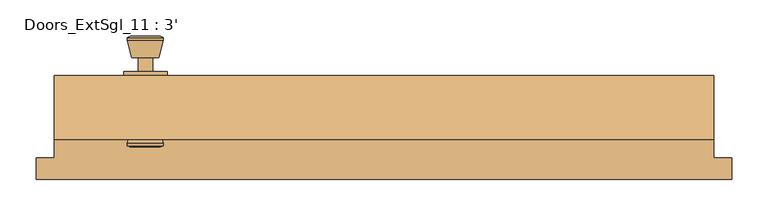
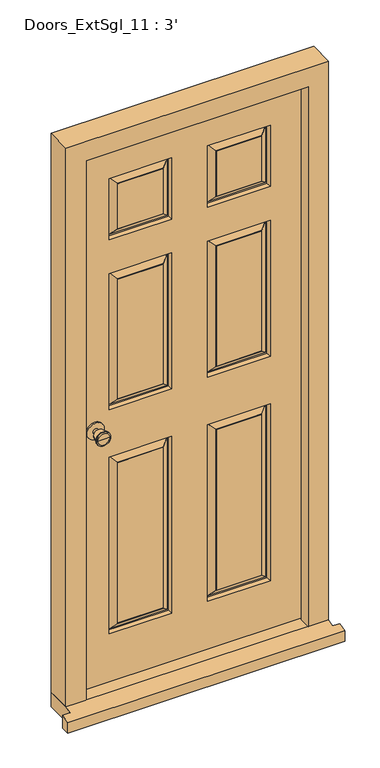
"""IFC4 building model written with IfcOpenShell, lengths in millimetres: door geometry, Doors_ExtSgl_11 : 3'."""

from ifc_helpers import new_model, si_unit, point, frame, frame_2d, origin, place, context, project, spatial, polyline, circle_curve, trimmed, segment, composite_curve, outline, extrude, faceted_brep, source, transform, mapped, element, save
from ifc_brep_helpers import plane_surface, cylinder_surface, revolved_surface, advanced_brep


def doors_extsgl_11_3_1bca8958(model_context):
    return source(origin(), model_context, "Body", "SolidModel", [
        advanced_brep(
        [(-330.7, 51.42, 1000.0), (-340.7, 51.42, 1000.0), (-320.7, 51.42, 1000.0), (-310.2241324, 100.42, 1000.0), (-351.1758676, 100.42, 1000.0), (-330.7, 100.42, 1000.0), (-305.7, 98.5921319, 1000.0), (-355.7, 98.5921319, 1000.0), (-305.7, 95.1284537, 1000.0), (-355.7, 95.1284537, 1000.0), (-312.063764, 70.42, 1000.0), (-349.336236, 70.42, 1000.0), (-320.7, 70.42, 1000.0), (-340.7, 70.42, 1000.0)],
        [
            (0, 1),
            (1, 2, circle_curve(frame((-330.7, 51.42, 1000.0), z_axis=(0.0, -1.0, 0.0), x_axis=(-1.0, 0.0, 0.0)), 10.0)),
            (2, 0),
            (2, 1, circle_curve(frame((-330.7, 51.42, 1000.0), z_axis=(0.0, -1.0, 0.0), x_axis=(-1.0, 0.0, 0.0)), 10.0)),
            (3, 4, circle_curve(frame((-330.7, 100.42, 1000.0), z_axis=(0.0, 1.0, 0.0), x_axis=(-1.0, 0.0, 0.0)), 20.4758676)),
            (4, 5),
            (5, 3),
            (4, 3, circle_curve(frame((-330.7, 100.42, 1000.0), z_axis=(0.0, 1.0, 0.0), x_axis=(-1.0, 0.0, 0.0)), 20.4758676)),
            (6, 7, circle_curve(frame((-330.7, 98.5921319, 1000.0), z_axis=(0.0, 1.0, 0.0), x_axis=(-1.0, 0.0, 0.0)), 25.0)),
            (7, 4),
            (3, 6),
            (7, 6, circle_curve(frame((-330.7, 98.5921319, 1000.0), z_axis=(0.0, 1.0, 0.0), x_axis=(-1.0, 0.0, 0.0)), 25.0)),
            (8, 9, circle_curve(frame((-330.7, 95.1284537, 1000.0), z_axis=(0.0, 1.0, 0.0), x_axis=(-1.0, 0.0, 0.0)), 25.0)),
            (9, 7),
            (6, 8),
            (9, 8, circle_curve(frame((-330.7, 95.1284537, 1000.0), z_axis=(0.0, 1.0, 0.0), x_axis=(-1.0, 0.0, 0.0)), 25.0)),
            (10, 11, circle_curve(frame((-330.7, 70.42, 1000.0), z_axis=(0.0, 1.0, 0.0), x_axis=(-1.0, 0.0, 0.0)), 18.636236)),
            (11, 9),
            (8, 10),
            (11, 10, circle_curve(frame((-330.7, 70.42, 1000.0), z_axis=(0.0, 1.0, 0.0), x_axis=(-1.0, 0.0, 0.0)), 18.636236)),
            (12, 13, circle_curve(frame((-330.7, 70.42, 1000.0), z_axis=(0.0, 1.0, 0.0), x_axis=(-1.0, 0.0, 0.0)), 10.0)),
            (13, 11),
            (10, 12),
            (13, 12, circle_curve(frame((-330.7, 70.42, 1000.0), z_axis=(0.0, 1.0, 0.0), x_axis=(-1.0, 0.0, 0.0)), 10.0)),
            (1, 13),
            (12, 2),
        ],
        [
            plane_surface(frame((-330.7, 51.42, 1000.0), z_axis=(0.0, -1.0, 0.0), x_axis=(-1.0, 0.0, 0.0))),
            plane_surface(frame((-330.7, 100.42, 1000.0), z_axis=(0.0, 1.0, 0.0), x_axis=(-1.0, 0.0, 0.0))),
            revolved_surface(polyline([(-351.1758676, 100.42, 1000.0), (-355.7, 98.5921319, 1000.0)]), (-330.7, 51.42, 1000.0), (0.0, -1.0, 0.0)),
            cylinder_surface(frame((-330.7, 51.42, 1000.0), z_axis=(0.0, -1.0, 0.0), x_axis=(-1.0, 0.0, 0.0)), 25.0),
            revolved_surface(polyline([(-355.7, 95.1284537, 1000.0), (-349.336236, 70.42, 1000.0)]), (-330.7, 51.42, 1000.0), (0.0, -1.0, 0.0)),
            plane_surface(frame((-330.7, 70.42, 1000.0), z_axis=(0.0, -1.0, 0.0), x_axis=(-1.0, 0.0, 0.0))),
            cylinder_surface(frame((-330.7, 51.42, 1000.0), z_axis=(0.0, -1.0, 0.0), x_axis=(-1.0, 0.0, 0.0)), 10.0),
        ],
        [
            (0, [[1, 2, 3]]),
            (0, [[-3, 4, -1]]),
            (1, [[5, 6, 7]]),
            (1, [[8, -7, -6]]),
            (2, [[9, 10, -5, 11]]),
            (2, [[12, -11, -8, -10]]),
            (3, [[13, 14, -9, 15]]),
            (3, [[16, -15, -12, -14]]),
            (4, [[17, 18, -13, 19]]),
            (4, [[20, -19, -16, -18]]),
            (5, [[21, 22, -17, 23]]),
            (5, [[24, -23, -20, -22]]),
            (6, [[-2, 25, -21, 26]]),
            (6, [[-4, -26, -24, -25]]),
        ],
    ),
        extrude(outline(composite_curve([segment(trimmed(circle_curve(frame_2d((1000.0, -330.7)), 30.0), [point((1000.0, -360.7))], [point((1000.0, -300.7))], False, "CARTESIAN"), True, "CONTINUOUS"), segment(trimmed(circle_curve(frame_2d((1000.0, -330.7)), 30.0), [point((1000.0, -300.7))], [point((1000.0, -360.7))], False, "CARTESIAN"), True, "CONTINUOUS")], self_intersect=False)), frame((0.0, 45.42, 0.0), z_axis=(0.0, 1.0, 0.0), x_axis=(0.0, 0.0, 1.0)), (0.0, 0.0, 1.0), 6.0),
        advanced_brep(
        [(-330.7, -4.58, 1000.0), (-320.7, -4.58, 1000.0), (-340.7, -4.58, 1000.0), (-310.2241324, -53.58, 1000.0), (-330.7, -53.58, 1000.0), (-351.1758676, -53.58, 1000.0), (-305.7, -51.7521319, 1000.0), (-355.7, -51.7521319, 1000.0), (-305.7, -48.2884537, 1000.0), (-355.7, -48.2884537, 1000.0), (-312.063764, -23.58, 1000.0), (-349.336236, -23.58, 1000.0), (-320.7, -23.58, 1000.0), (-340.7, -23.58, 1000.0)],
        [
            (0, 1),
            (1, 2, circle_curve(frame((-330.7, -4.58, 1000.0), z_axis=(0.0, 1.0, 0.0), x_axis=(-1.0, 0.0, 0.0)), 10.0)),
            (2, 0),
            (2, 1, circle_curve(frame((-330.7, -4.58, 1000.0), z_axis=(0.0, 1.0, 0.0), x_axis=(-1.0, 0.0, 0.0)), 10.0)),
            (3, 4),
            (4, 5),
            (5, 3, circle_curve(frame((-330.7, -53.58, 1000.0), z_axis=(0.0, -1.0, 0.0), x_axis=(-1.0, 0.0, 0.0)), 20.4758676)),
            (3, 5, circle_curve(frame((-330.7, -53.58, 1000.0), z_axis=(0.0, -1.0, 0.0), x_axis=(-1.0, 0.0, 0.0)), 20.4758676)),
            (6, 3),
            (5, 7),
            (7, 6, circle_curve(frame((-330.7, -51.7521319, 1000.0), z_axis=(0.0, -1.0, 0.0), x_axis=(-1.0, 0.0, 0.0)), 25.0)),
            (6, 7, circle_curve(frame((-330.7, -51.7521319, 1000.0), z_axis=(0.0, -1.0, 0.0), x_axis=(-1.0, 0.0, 0.0)), 25.0)),
            (8, 6),
            (7, 9),
            (9, 8, circle_curve(frame((-330.7, -48.2884537, 1000.0), z_axis=(0.0, -1.0, 0.0), x_axis=(-1.0, 0.0, 0.0)), 25.0)),
            (8, 9, circle_curve(frame((-330.7, -48.2884537, 1000.0), z_axis=(0.0, -1.0, 0.0), x_axis=(-1.0, 0.0, 0.0)), 25.0)),
            (10, 8),
            (9, 11),
            (11, 10, circle_curve(frame((-330.7, -23.58, 1000.0), z_axis=(0.0, -1.0, 0.0), x_axis=(-1.0, 0.0, 0.0)), 18.636236)),
            (10, 11, circle_curve(frame((-330.7, -23.58, 1000.0), z_axis=(0.0, -1.0, 0.0), x_axis=(-1.0, 0.0, 0.0)), 18.636236)),
            (12, 10),
            (11, 13),
            (13, 12, circle_curve(frame((-330.7, -23.58, 1000.0), z_axis=(0.0, -1.0, 0.0), x_axis=(-1.0, 0.0, 0.0)), 10.0)),
            (12, 13, circle_curve(frame((-330.7, -23.58, 1000.0), z_axis=(0.0, -1.0, 0.0), x_axis=(-1.0, 0.0, 0.0)), 10.0)),
            (1, 12),
            (13, 2),
        ],
        [
            plane_surface(frame((-330.7, -4.58, 1000.0), z_axis=(0.0, 1.0, 0.0), x_axis=(-1.0, 0.0, 0.0))),
            plane_surface(frame((-330.7, -53.58, 1000.0), z_axis=(0.0, -1.0, 0.0), x_axis=(-1.0, 0.0, 0.0))),
            revolved_surface(polyline([(-351.1758676, -53.58, 1000.0), (-355.7, -51.7521319, 1000.0)]), (-330.7, -4.58, 1000.0), (0.0, 1.0, 0.0)),
            cylinder_surface(frame((-330.7, -4.58, 1000.0), z_axis=(0.0, 1.0, 0.0), x_axis=(-1.0, 0.0, 0.0)), 25.0),
            revolved_surface(polyline([(-355.7, -48.2884537, 1000.0), (-349.336236, -23.58, 1000.0)]), (-330.7, -4.58, 1000.0), (0.0, 1.0, 0.0)),
            plane_surface(frame((-330.7, -23.58, 1000.0), z_axis=(0.0, 1.0, 0.0), x_axis=(-1.0, 0.0, 0.0))),
            cylinder_surface(frame((-330.7, -4.58, 1000.0), z_axis=(0.0, 1.0, 0.0), x_axis=(-1.0, 0.0, 0.0)), 10.0),
        ],
        [
            (0, [[1, 2, 3]]),
            (0, [[-3, 4, -1]]),
            (1, [[5, 6, 7]]),
            (1, [[-6, -5, 8]]),
            (2, [[9, -7, 10, 11]]),
            (2, [[-10, -8, -9, 12]]),
            (3, [[13, -11, 14, 15]]),
            (3, [[-14, -12, -13, 16]]),
            (4, [[17, -15, 18, 19]]),
            (4, [[-18, -16, -17, 20]]),
            (5, [[21, -19, 22, 23]]),
            (5, [[-22, -20, -21, 24]]),
            (6, [[25, -23, 26, -2]]),
            (6, [[-26, -24, -25, -4]]),
        ],
    ),
        extrude(outline(composite_curve([segment(trimmed(circle_curve(frame_2d((1000.0, -330.7)), 30.0), [point((1000.0, -360.7))], [point((1000.0, -300.7))], False, "CARTESIAN"), True, "CONTINUOUS"), segment(trimmed(circle_curve(frame_2d((1000.0, -330.7)), 30.0), [point((1000.0, -300.7))], [point((1000.0, -360.7))], False, "CARTESIAN"), True, "CONTINUOUS")], self_intersect=False)), frame((0.0, -4.58, 0.0), z_axis=(0.0, 1.0, 0.0), x_axis=(0.0, 0.0, 1.0)), (0.0, 0.0, 1.0), 6.0),
        faceted_brep([(386.7, -43.58, 54.5), (386.7, -1.58, 54.5), (408.7, -1.58, 54.5), (408.7, 45.42, 54.5), (457.2, 45.42, 54.5), (457.2, -43.58, 54.5), (457.2, -43.58, 2110.0), (-457.2, -43.58, 2110.0), (-457.2, -43.58, 54.5), (-386.7, -43.58, 54.5), (-386.7, -43.58, 2039.5), (386.7, -43.58, 2039.5), (457.2, 45.42, 2110.0), (408.7, 45.42, 2061.5), (-408.7, 45.42, 2061.5), (-408.7, 45.42, 54.5), (-457.2, 45.42, 54.5), (-457.2, 45.42, 2110.0), (408.7, -1.58, 2061.5), (386.7, -1.58, 2039.5), (-386.7, -1.58, 2039.5), (-386.7, -1.58, 54.5), (-408.7, -1.58, 54.5), (-408.7, -1.58, 2061.5)], [[[0, 1, 2, 3, 4, 5]], [[5, 6, 7, 8, 9, 10, 11, 0]], [[4, 12, 6, 5]], [[3, 13, 14, 15, 16, 17, 12, 4]], [[2, 18, 13, 3]], [[1, 19, 20, 21, 22, 23, 18, 2]], [[0, 11, 19, 1]], [[9, 21, 20, 10]], [[8, 16, 15, 22, 21, 9]], [[7, 17, 16, 8]], [[14, 23, 22, 15]], [[6, 12, 17, 7]], [[13, 18, 23, 14]], [[10, 20, 19, 11]]]),
        faceted_brep([(405.7, 45.42, 58.5), (-406.6250294, 45.42, 58.5), (-406.6250294, 45.42, 2058.5), (405.7, 45.42, 2058.5), (-62.5, 45.42, 883.5), (-280.7, 45.42, 883.5), (-280.7, 45.42, 233.5), (-62.5, 45.42, 233.5), (280.7, 45.42, 883.5), (62.5, 45.42, 883.5), (62.5, 45.42, 233.5), (280.7, 45.42, 233.5), (-62.5, 45.42, 1558.5), (-280.7, 45.42, 1558.5), (-280.7, 45.42, 1058.5), (-62.5, 45.42, 1058.5), (280.7, 45.42, 1558.5), (62.5, 45.42, 1558.5), (62.5, 45.42, 1058.5), (280.7, 45.42, 1058.5), (-62.5, 45.42, 1908.5), (-280.7, 45.42, 1908.5), (-280.7, 45.42, 1683.5), (-62.5, 45.42, 1683.5), (62.5, 45.42, 1683.5), (280.7, 45.42, 1683.5), (280.7, 45.42, 1908.5), (62.5, 45.42, 1908.5), (-92.5, 45.42, 263.5), (-250.7, 45.42, 263.5), (-250.7, 45.42, 853.5), (-92.5, 45.42, 853.5), (250.7, 45.42, 263.5), (92.5, 45.42, 263.5), (92.5, 45.42, 853.5), (250.7, 45.42, 853.5), (-92.5, 45.42, 1088.5), (-250.7, 45.42, 1088.5), (-250.7, 45.42, 1528.5), (-92.5, 45.42, 1528.5), (250.7, 45.42, 1088.5), (92.5, 45.42, 1088.5), (92.5, 45.42, 1528.5), (250.7, 45.42, 1528.5), (-92.5, 45.42, 1713.5), (-250.7, 45.42, 1713.5), (-250.7, 45.42, 1878.5), (-92.5, 45.42, 1878.5), (92.5, 45.42, 1878.5), (250.7, 45.42, 1878.5), (250.7, 45.42, 1713.5), (92.5, 45.42, 1713.5), (405.7, 1.42, 58.5), (405.7, 1.42, 2058.5), (-406.6250294, 1.42, 2058.5), (-406.6250294, 1.42, 58.5), (62.5, 1.42, 883.5), (280.7, 1.42, 883.5), (280.7, 1.42, 233.5), (62.5, 1.42, 233.5), (-280.7, 1.42, 883.5), (-62.5, 1.42, 883.5), (-62.5, 1.42, 233.5), (-280.7, 1.42, 233.5), (62.5, 1.42, 1558.5), (280.7, 1.42, 1558.5), (280.7, 1.42, 1058.5), (62.5, 1.42, 1058.5), (-280.7, 1.42, 1558.5), (-62.5, 1.42, 1558.5), (-62.5, 1.42, 1058.5), (-280.7, 1.42, 1058.5), (62.5, 1.42, 1908.5), (280.7, 1.42, 1908.5), (280.7, 1.42, 1683.5), (62.5, 1.42, 1683.5), (-280.7, 1.42, 1908.5), (-62.5, 1.42, 1908.5), (-62.5, 1.42, 1683.5), (-280.7, 1.42, 1683.5), (92.5, 1.42, 263.5), (250.7, 1.42, 263.5), (250.7, 1.42, 853.5), (92.5, 1.42, 853.5), (-250.7, 1.42, 263.5), (-92.5, 1.42, 263.5), (-92.5, 1.42, 853.5), (-250.7, 1.42, 853.5), (92.5, 1.42, 1088.5), (250.7, 1.42, 1088.5), (250.7, 1.42, 1528.5), (92.5, 1.42, 1528.5), (-250.7, 1.42, 1088.5), (-92.5, 1.42, 1088.5), (-92.5, 1.42, 1528.5), (-250.7, 1.42, 1528.5), (92.5, 1.42, 1713.5), (250.7, 1.42, 1713.5), (250.7, 1.42, 1878.5), (92.5, 1.42, 1878.5), (-250.7, 1.42, 1713.5), (-92.5, 1.42, 1713.5), (-92.5, 1.42, 1878.5), (-250.7, 1.42, 1878.5), (65.5, 16.42, 880.5), (65.5, 16.42, 236.5), (90.5, 2.42, 855.5), (70.5, 16.42, 875.5), (70.5, 16.42, 241.5), (90.5, 2.42, 261.5), (92.5, 2.42, 853.5), (92.5, 2.42, 263.5), (277.7, 16.42, 236.5), (272.7, 16.42, 241.5), (252.7, 2.42, 261.5), (250.7, 2.42, 263.5), (277.7, 16.42, 880.5), (272.7, 16.42, 875.5), (252.7, 2.42, 855.5), (250.7, 2.42, 853.5), (-277.7, 16.42, 880.5), (-277.7, 16.42, 236.5), (-252.7, 2.42, 855.5), (-272.7, 16.42, 875.5), (-272.7, 16.42, 241.5), (-252.7, 2.42, 261.5), (-250.7, 2.42, 853.5), (-250.7, 2.42, 263.5), (-65.5, 16.42, 236.5), (-70.5, 16.42, 241.5), (-90.5, 2.42, 261.5), (-92.5, 2.42, 263.5), (-65.5, 16.42, 880.5), (-70.5, 16.42, 875.5), (-90.5, 2.42, 855.5), (-92.5, 2.42, 853.5), (-92.5, 44.42, 263.5), (-92.5, 44.42, 853.5), (-70.5, 30.42, 241.5), (-90.5, 44.42, 261.5), (-90.5, 44.42, 855.5), (-70.5, 30.42, 875.5), (-65.5, 30.42, 236.5), (-65.5, 30.42, 880.5), (-250.7, 44.42, 853.5), (-252.7, 44.42, 855.5), (-272.7, 30.42, 875.5), (-277.7, 30.42, 880.5), (-250.7, 44.42, 263.5), (-252.7, 44.42, 261.5), (-272.7, 30.42, 241.5), (-277.7, 30.42, 236.5), (277.7, 30.42, 880.5), (277.7, 30.42, 236.5), (252.7, 44.42, 855.5), (272.7, 30.42, 875.5), (272.7, 30.42, 241.5), (252.7, 44.42, 261.5), (250.7, 44.42, 853.5), (250.7, 44.42, 263.5), (65.5, 30.42, 236.5), (70.5, 30.42, 241.5), (90.5, 44.42, 261.5), (92.5, 44.42, 263.5), (65.5, 30.42, 880.5), (70.5, 30.42, 875.5), (90.5, 44.42, 855.5), (92.5, 44.42, 853.5), (92.5, 2.42, 1088.5), (92.5, 2.42, 1528.5), (70.5, 16.42, 1066.5), (90.5, 2.42, 1086.5), (90.5, 2.42, 1530.5), (70.5, 16.42, 1550.5), (65.5, 16.42, 1061.5), (65.5, 16.42, 1555.5), (250.7, 2.42, 1528.5), (252.7, 2.42, 1530.5), (272.7, 16.42, 1550.5), (277.7, 16.42, 1555.5), (250.7, 2.42, 1088.5), (252.7, 2.42, 1086.5), (272.7, 16.42, 1066.5), (277.7, 16.42, 1061.5), (-250.7, 2.42, 1088.5), (-250.7, 2.42, 1528.5), (-272.7, 16.42, 1066.5), (-252.7, 2.42, 1086.5), (-252.7, 2.42, 1530.5), (-272.7, 16.42, 1550.5), (-277.7, 16.42, 1061.5), (-277.7, 16.42, 1555.5), (-92.5, 2.42, 1528.5), (-90.5, 2.42, 1530.5), (-70.5, 16.42, 1550.5), (-65.5, 16.42, 1555.5), (-92.5, 2.42, 1088.5), (-90.5, 2.42, 1086.5), (-70.5, 16.42, 1066.5), (-65.5, 16.42, 1061.5), (-92.5, 44.42, 1088.5), (-92.5, 44.42, 1528.5), (-70.5, 30.42, 1066.5), (-90.5, 44.42, 1086.5), (-90.5, 44.42, 1530.5), (-70.5, 30.42, 1550.5), (-65.5, 30.42, 1061.5), (-65.5, 30.42, 1555.5), (-250.7, 44.42, 1528.5), (-252.7, 44.42, 1530.5), (-272.7, 30.42, 1550.5), (-277.7, 30.42, 1555.5), (-250.7, 44.42, 1088.5), (-252.7, 44.42, 1086.5), (-272.7, 30.42, 1066.5), (-277.7, 30.42, 1061.5), (277.7, 30.42, 1555.5), (277.7, 30.42, 1061.5), (252.7, 44.42, 1530.5), (272.7, 30.42, 1550.5), (272.7, 30.42, 1066.5), (252.7, 44.42, 1086.5), (250.7, 44.42, 1528.5), (250.7, 44.42, 1088.5), (65.5, 30.42, 1061.5), (70.5, 30.42, 1066.5), (90.5, 44.42, 1086.5), (92.5, 44.42, 1088.5), (65.5, 30.42, 1555.5), (70.5, 30.42, 1550.5), (90.5, 44.42, 1530.5), (92.5, 44.42, 1528.5), (92.5, 2.42, 1713.5), (92.5, 2.42, 1878.5), (70.5, 16.42, 1691.5), (90.5, 2.42, 1711.5), (90.5, 2.42, 1880.5), (70.5, 16.42, 1900.5), (65.5, 16.42, 1686.5), (65.5, 16.42, 1905.5), (250.7, 2.42, 1878.5), (252.7, 2.42, 1880.5), (272.7, 16.42, 1900.5), (277.7, 16.42, 1905.5), (250.7, 2.42, 1713.5), (252.7, 2.42, 1711.5), (272.7, 16.42, 1691.5), (277.7, 16.42, 1686.5), (-250.7, 2.42, 1713.5), (-250.7, 2.42, 1878.5), (-272.7, 16.42, 1691.5), (-252.7, 2.42, 1711.5), (-252.7, 2.42, 1880.5), (-272.7, 16.42, 1900.5), (-277.7, 16.42, 1686.5), (-277.7, 16.42, 1905.5), (-92.5, 2.42, 1878.5), (-90.5, 2.42, 1880.5), (-70.5, 16.42, 1900.5), (-65.5, 16.42, 1905.5), (-92.5, 2.42, 1713.5), (-90.5, 2.42, 1711.5), (-70.5, 16.42, 1691.5), (-65.5, 16.42, 1686.5), (-92.5, 44.42, 1713.5), (-92.5, 44.42, 1878.5), (-70.5, 30.42, 1691.5), (-90.5, 44.42, 1711.5), (-90.5, 44.42, 1880.5), (-70.5, 30.42, 1900.5), (-65.5, 30.42, 1686.5), (-65.5, 30.42, 1905.5), (-250.7, 44.42, 1878.5), (-252.7, 44.42, 1880.5), (-272.7, 30.42, 1900.5), (-277.7, 30.42, 1905.5), (-250.7, 44.42, 1713.5), (-252.7, 44.42, 1711.5), (-272.7, 30.42, 1691.5), (-277.7, 30.42, 1686.5), (92.5, 44.42, 1878.5), (92.5, 44.42, 1713.5), (70.5, 30.42, 1900.5), (90.5, 44.42, 1880.5), (90.5, 44.42, 1711.5), (70.5, 30.42, 1691.5), (65.5, 30.42, 1905.5), (65.5, 30.42, 1686.5), (250.7, 44.42, 1713.5), (252.7, 44.42, 1711.5), (272.7, 30.42, 1691.5), (277.7, 30.42, 1686.5), (250.7, 44.42, 1878.5), (252.7, 44.42, 1880.5), (272.7, 30.42, 1900.5), (277.7, 30.42, 1905.5)], [[[0, 1, 2, 3], [4, 5, 6, 7], [8, 9, 10, 11], [12, 13, 14, 15], [16, 17, 18, 19], [20, 21, 22, 23], [24, 25, 26, 27]], [[28, 29, 30, 31]], [[32, 33, 34, 35]], [[36, 37, 38, 39]], [[40, 41, 42, 43]], [[44, 45, 46, 47]], [[48, 49, 50, 51]], [[52, 53, 54, 55], [56, 57, 58, 59], [60, 61, 62, 63], [64, 65, 66, 67], [68, 69, 70, 71], [72, 73, 74, 75], [76, 77, 78, 79]], [[80, 81, 82, 83]], [[84, 85, 86, 87]], [[88, 89, 90, 91]], [[92, 93, 94, 95]], [[96, 97, 98, 99]], [[100, 101, 102, 103]], [[3, 53, 52, 0]], [[2, 54, 53, 3]], [[1, 55, 54, 2]], [[0, 52, 55, 1]], [[104, 56, 59, 105]], [[106, 107, 108, 109]], [[80, 83, 110, 111]], [[59, 58, 112, 105]], [[108, 113, 114, 109]], [[111, 115, 81, 80]], [[58, 57, 116, 112]], [[113, 117, 118, 114]], [[115, 119, 82, 81]], [[104, 116, 57, 56]], [[105, 112, 116, 104], [107, 117, 113, 108]], [[106, 118, 117, 107]], [[109, 114, 118, 106], [110, 119, 115, 111]], [[83, 82, 119, 110]], [[120, 60, 63, 121]], [[122, 123, 124, 125]], [[84, 87, 126, 127]], [[63, 62, 128, 121]], [[124, 129, 130, 125]], [[127, 131, 85, 84]], [[62, 61, 132, 128]], [[129, 133, 134, 130]], [[131, 135, 86, 85]], [[120, 132, 61, 60]], [[121, 128, 132, 120], [123, 133, 129, 124]], [[122, 134, 133, 123]], [[125, 130, 134, 122], [126, 135, 131, 127]], [[87, 86, 135, 126]], [[136, 28, 31, 137]], [[138, 139, 140, 141]], [[4, 7, 142, 143]], [[31, 30, 144, 137]], [[140, 145, 146, 141]], [[143, 147, 5, 4]], [[30, 29, 148, 144]], [[145, 149, 150, 146]], [[147, 151, 6, 5]], [[136, 148, 29, 28]], [[139, 149, 145, 140], [137, 144, 148, 136]], [[138, 150, 149, 139]], [[142, 151, 147, 143], [141, 146, 150, 138]], [[7, 6, 151, 142]], [[152, 8, 11, 153]], [[154, 155, 156, 157]], [[32, 35, 158, 159]], [[11, 10, 160, 153]], [[156, 161, 162, 157]], [[159, 163, 33, 32]], [[10, 9, 164, 160]], [[161, 165, 166, 162]], [[163, 167, 34, 33]], [[152, 164, 9, 8]], [[153, 160, 164, 152], [155, 165, 161, 156]], [[154, 166, 165, 155]], [[157, 162, 166, 154], [158, 167, 163, 159]], [[35, 34, 167, 158]], [[168, 88, 91, 169]], [[170, 171, 172, 173]], [[64, 67, 174, 175]], [[91, 90, 176, 169]], [[172, 177, 178, 173]], [[175, 179, 65, 64]], [[90, 89, 180, 176]], [[177, 181, 182, 178]], [[179, 183, 66, 65]], [[168, 180, 89, 88]], [[171, 181, 177, 172], [169, 176, 180, 168]], [[170, 182, 181, 171]], [[174, 183, 179, 175], [173, 178, 182, 170]], [[67, 66, 183, 174]], [[184, 92, 95, 185]], [[186, 187, 188, 189]], [[68, 71, 190, 191]], [[95, 94, 192, 185]], [[188, 193, 194, 189]], [[191, 195, 69, 68]], [[94, 93, 196, 192]], [[193, 197, 198, 194]], [[195, 199, 70, 69]], [[184, 196, 93, 92]], [[187, 197, 193, 188], [185, 192, 196, 184]], [[186, 198, 197, 187]], [[190, 199, 195, 191], [189, 194, 198, 186]], [[71, 70, 199, 190]], [[200, 36, 39, 201]], [[202, 203, 204, 205]], [[12, 15, 206, 207]], [[39, 38, 208, 201]], [[204, 209, 210, 205]], [[207, 211, 13, 12]], [[38, 37, 212, 208]], [[209, 213, 214, 210]], [[211, 215, 14, 13]], [[200, 212, 37, 36]], [[203, 213, 209, 204], [201, 208, 212, 200]], [[202, 214, 213, 203]], [[206, 215, 211, 207], [205, 210, 214, 202]], [[15, 14, 215, 206]], [[216, 16, 19, 217]], [[218, 219, 220, 221]], [[40, 43, 222, 223]], [[19, 18, 224, 217]], [[220, 225, 226, 221]], [[223, 227, 41, 40]], [[18, 17, 228, 224]], [[225, 229, 230, 226]], [[227, 231, 42, 41]], [[216, 228, 17, 16]], [[217, 224, 228, 216], [219, 229, 225, 220]], [[218, 230, 229, 219]], [[221, 226, 230, 218], [222, 231, 227, 223]], [[43, 42, 231, 222]], [[232, 96, 99, 233]], [[234, 235, 236, 237]], [[72, 75, 238, 239]], [[99, 98, 240, 233]], [[236, 241, 242, 237]], [[239, 243, 73, 72]], [[98, 97, 244, 240]], [[241, 245, 246, 242]], [[243, 247, 74, 73]], [[232, 244, 97, 96]], [[235, 245, 241, 236], [233, 240, 244, 232]], [[234, 246, 245, 235]], [[238, 247, 243, 239], [237, 242, 246, 234]], [[75, 74, 247, 238]], [[248, 100, 103, 249]], [[250, 251, 252, 253]], [[76, 79, 254, 255]], [[103, 102, 256, 249]], [[252, 257, 258, 253]], [[255, 259, 77, 76]], [[102, 101, 260, 256]], [[257, 261, 262, 258]], [[259, 263, 78, 77]], [[248, 260, 101, 100]], [[251, 261, 257, 252], [249, 256, 260, 248]], [[250, 262, 261, 251]], [[254, 263, 259, 255], [253, 258, 262, 250]], [[79, 78, 263, 254]], [[264, 44, 47, 265]], [[266, 267, 268, 269]], [[20, 23, 270, 271]], [[47, 46, 272, 265]], [[268, 273, 274, 269]], [[271, 275, 21, 20]], [[46, 45, 276, 272]], [[273, 277, 278, 274]], [[275, 279, 22, 21]], [[264, 276, 45, 44]], [[267, 277, 273, 268], [265, 272, 276, 264]], [[266, 278, 277, 267]], [[270, 279, 275, 271], [269, 274, 278, 266]], [[23, 22, 279, 270]], [[280, 48, 51, 281]], [[282, 283, 284, 285]], [[24, 27, 286, 287]], [[51, 50, 288, 281]], [[284, 289, 290, 285]], [[287, 291, 25, 24]], [[50, 49, 292, 288]], [[289, 293, 294, 290]], [[291, 295, 26, 25]], [[280, 292, 49, 48]], [[283, 293, 289, 284], [281, 288, 292, 280]], [[282, 294, 293, 283]], [[286, 295, 291, 287], [285, 290, 294, 282]], [[27, 26, 295, 286]]]),
        faceted_brep([(482.2, -98.58, 0.0), (482.2, -68.58, 0.0), (482.2, -68.58, 47.2703282), (482.2, -98.58, 38.5947221), (-482.2, -98.58, 38.5947221), (-482.2, -68.58, 47.2703282), (-482.2, -68.58, 0.0), (-482.2, -98.58, 0.0), (-457.2, -68.58, 0.0), (-457.2, 45.42, 0.0), (457.2, 45.42, 0.0), (457.2, -68.58, 0.0), (457.2, -68.58, 47.2703282), (457.2, -43.58, 54.5), (-457.2, -43.58, 54.5), (-457.2, -68.58, 47.2703282), (457.2, 45.42, 54.5), (-457.2, 45.42, 54.5)], [[[0, 1, 2, 3]], [[4, 5, 6, 7]], [[7, 6, 8, 9, 10, 11, 1, 0]], [[3, 4, 7, 0]], [[3, 2, 12, 13, 14, 15, 5, 4]], [[14, 13, 16, 17]], [[17, 16, 10, 9]], [[15, 14, 17, 9, 8]], [[8, 6, 5, 15]], [[11, 10, 16, 13, 12]], [[12, 2, 1, 11]]]),
    ])


if __name__ == "__main__":
    model = new_model("IFC4")
    model_context = context("Model", 3, world=origin())
    ifc_project = project(units=[si_unit("LENGTHUNIT", "METRE", prefix="MILLI")], contexts=[model_context])
    site = spatial("IfcSite", under=ifc_project)
    building = spatial("IfcBuilding", under=site)
    placement = place(None, origin())
    doors_extsgl_11_3_shape = doors_extsgl_11_3_1bca8958(model_context)
    element("IfcDoor", 1, ObjectType="Doors_ExtSgl_11 : 3'", at=placement, inside=building, context=model_context, shape_type="MappedRepresentation", body=[
        mapped(doors_extsgl_11_3_shape, transform((0.0, 0.0, 0.0), x_axis=(1.0, 0.0, 0.0), y_axis=(0.0, 1.0, 0.0), z_axis=(0.0, 0.0, 1.0))),
    ])
    save(model, "model.ifc")

# Revit data of these elements
# Type "Doors_ExtSgl_11 : 3'"
#   Type Mark = "49"
#   Type Comments = "External Single"
#   Operation = "SingleSwingRight"
#   Construction Type Id = "MDOOR"
#   Keynote = "L20"
#   Analytic Construction = "Metal"
#   Wrap Layers (Int) from Ext = 177.5 mm
#   Wrap Layers (Ext) from Ext = 102.5 mm
#   Thickness = 44 mm
#   Stile Top of Lock rail = 1000 mm
#   Stile Top of Frieze Rail = 1625 mm
#   Stile Top Rail = 150 mm
#   Stile Shutting = 125 mm
#   Stile Muntin Rail = 125 mm
#   Stile Lock Rail = 175 mm
#   Stile Intermediate/Frieze = 125 mm
#   Stile Hanging = 125 mm
#   Stile Bottom Rail = 175 mm
#   Rough Width = 914.4 mm
#   Rough Height = 2110 mm
#   O/A Frame Width = 64 mm
#   Heat Transfer Coefficient (U) = 3.7021 W/(m²·K)
#   Handle Z Distance = 1000 mm
#   Glazing Thickness = 24 mm
#   FrameWidth = 42 mm
#   FrameOffset - External = 25 mm
#   FrameDepth = 89 mm
#   Door Panel Width = 811.4 mm
#   Door Panel Thickness = 44 mm
#   Door Panel Height = 2000 mm
#   Cill Thickness = 54.5 mm
#   Handle X Distance = 75 mm
#   Height = 2110 mm
#   Structural Tolerance = 6.5 mm
#   Tolerance = 3 mm
#   Undercut = 4 mm
#   Width = 914.4 mm
#   Cill Projection = 30 mm
#   Cill Extension = 25 mm
#   Cavity Closer Width = 50 mm
#   Cavity Closer Offset from Ext = 102.5 mm
#   Cavity Closer Depth = 85 mm
#   Vis - Ironmongery = yes
#   Vis - Cavity Closers = yes
#   Define Thermal Properties by = 1
#   Function = 1
#   Material Door = Door - Panel
#   Material Frame = Door - Frame/Mullion
#   Material Ironmongery = Door - Handle
#   Visual Light Transmittance = 0
#   Solar Heat Gain Coefficient = 0
#   Wall Closure = (empty or 0)
# Element 1 (IfcDoor, "Doors_ExtSgl_11 : 3'")
#   Materials on its faces: "Door - Panel", "Door - Handle", "Door - Frame/Mullion"
# Materials
#   "Door - Panel": class "Wood", colour RGB 210 159 95, transparency 0, Keynote = "L20", Cost = 0
#   "Door - Frame/Mullion": class "Wood", colour RGB 212 179 113, transparency 0, Keynote = "L20", Cost = 0
#   "Door - Handle": colour RGB 0 0 0, transparency 0, Keynote = "P21", Cost = 0
